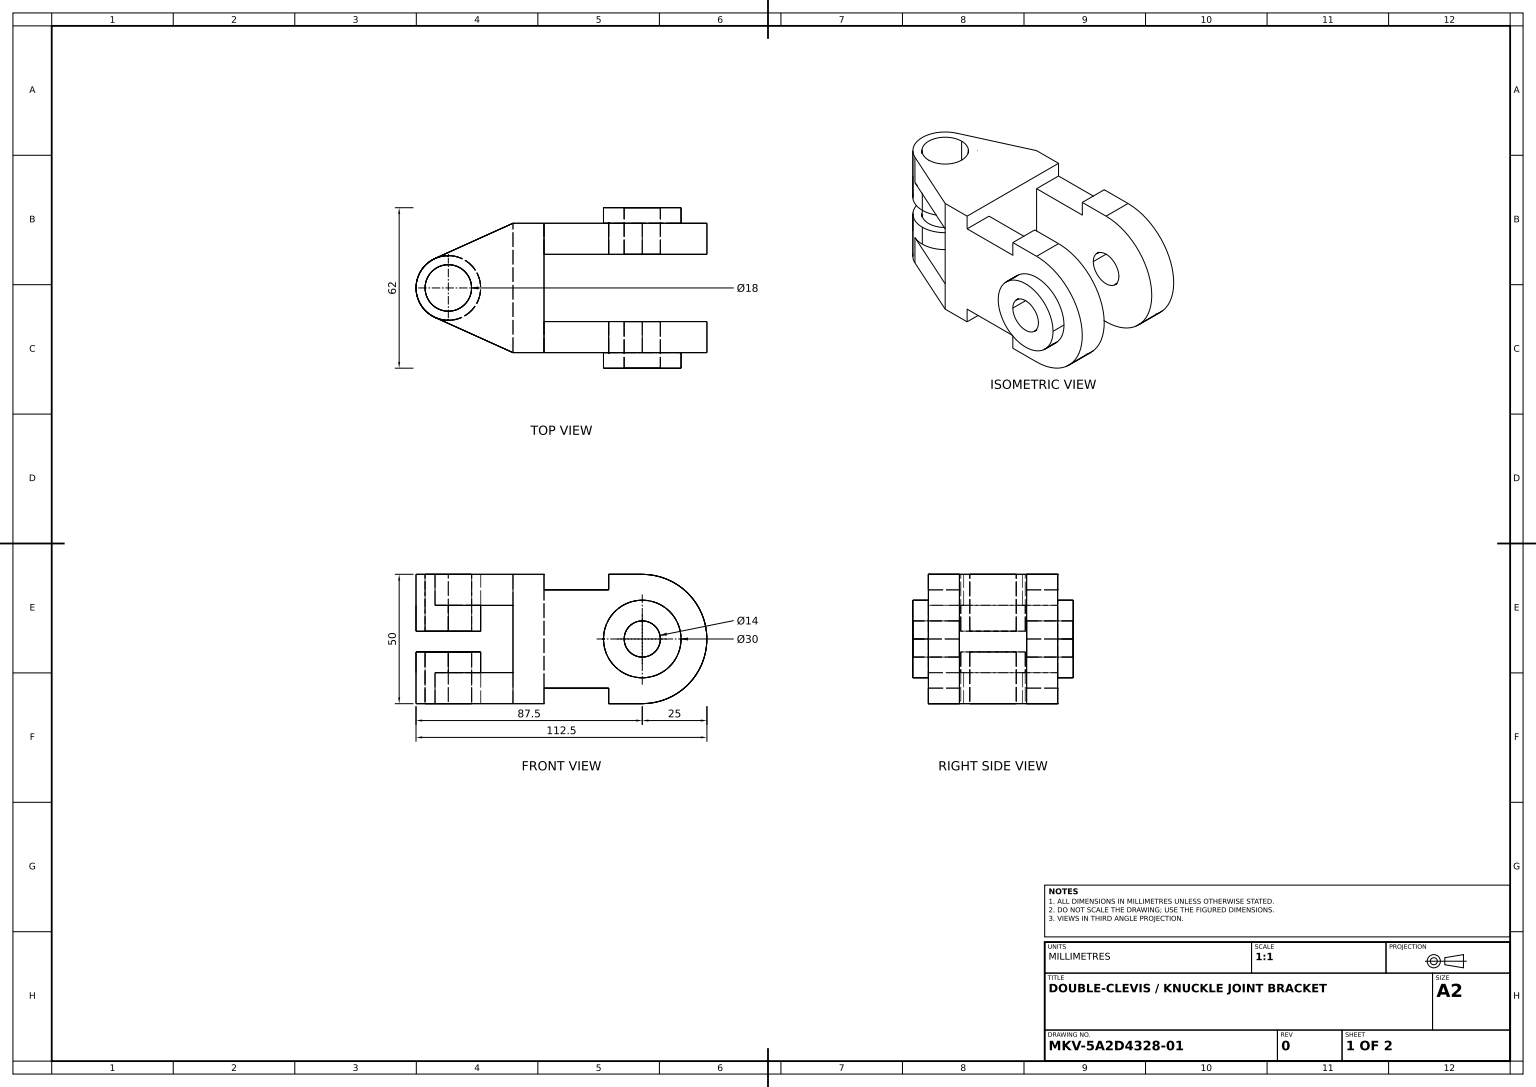
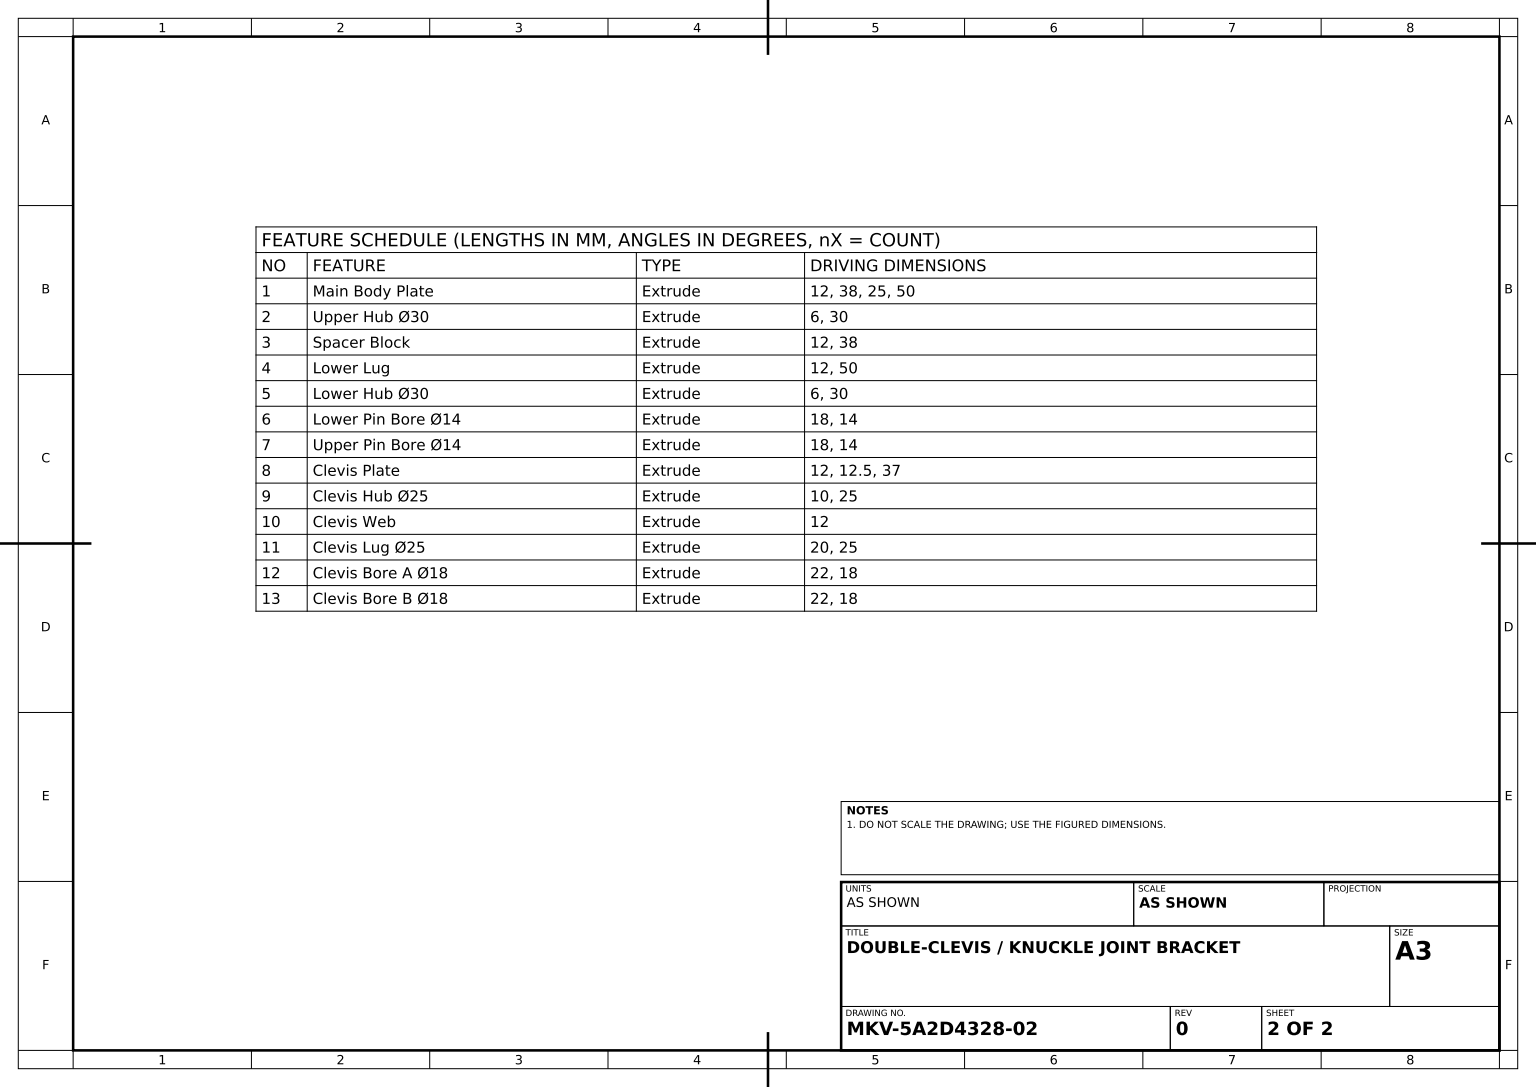
from build123d import *
from build123d.topology import SkipClean

# Parameters (mm, degrees)
MAIN_BODY_PLATE_DEPTH   = 12
UPPER_HUB_SKETCH_R      = 15
UPPER_HUB_30_DEPTH      = 6
SPACER_BLOCK_SKETCH_W   = 38
SPACER_BLOCK_SKETCH_H   = 50
SPACER_BLOCK_DEPTH      = 12
LOWER_LUG_DEPTH         = 12
LOWER_START             = 6
LOWER_HUB_SKETCH_R      = 15
LOWER_HUB_30_DEPTH      = 6
LOWER_PIN_BORE_SKETCH_R = 7
LOWER_PIN_BORE_14_DEPTH = 18
UPPER_START             = -18
UPPER_PIN_BORE_SKETCH_R = 7
UPPER_PIN_BORE_14_DEPTH = 18
CLEVIS_PLATE_DEPTH      = 12
CLEVIS_HUB_SKETCH_R     = 12.5
CLEVIS_HUB_25_DEPTH     = 10
CLEVIS_START            = -12
CLEVIS_WEB_DEPTH        = 12
CLEVIS_START_2          = -20
CLEVIS_LUG_SKETCH_R     = 12.5
CLEVIS_LUG_25_DEPTH     = 20
CLEVIS_BORE_A_SKETCH_R  = 9
CLEVIS_BORE_A_18_DEPTH  = 22
CLEVIS_START_3          = -22
CLEVIS_BORE_B_SKETCH_R  = 9
CLEVIS_BORE_B_18_DEPTH  = 22


with BuildPart() as part:
    # Main Body Profile Sketch → Main Body Plate (new body)
    with BuildSketch(Plane.XY):
        with BuildLine():
            Line((0, 0), (0, 50))
            Line((0, 50), (12, 50))
            Line((12, 50), (12, 44))
            Line((12, 44), (37, 44))
            Line((37, 44), (37, 50))
            Line((37, 50), (50, 50))
            ThreePointArc((50, 50), (75, 25), (50, 0))
            Line((50, 0), (37, 0))
            Line((37, 0), (37, 6))
            Line((37, 6), (12, 6))
            Line((12, 6), (12, 0))
            Line((12, 0), (0, 0))
        make_face()
    extrude(amount=MAIN_BODY_PLATE_DEPTH)

    # Upper Hub Sketch → Upper Hub Ø30 (add)
    with BuildSketch(Plane.XY.offset(12)):
        with Locations((50, 25)):
            Circle(UPPER_HUB_SKETCH_R)
    extrude(amount=UPPER_HUB_30_DEPTH)

    # Spacer Block Sketch → Spacer Block (add)
    with BuildSketch(Plane.ZY):
        with Locations((-19, 25)):
            Rectangle(SPACER_BLOCK_SKETCH_W, SPACER_BLOCK_SKETCH_H)
    extrude(amount=-SPACER_BLOCK_DEPTH)

    # Lower Lug Sketch → Lower Lug (add)
    with BuildSketch(Plane(origin=(0, 0, -38), x_dir=(-1, 0, 0), z_dir=(0, 0, -1))):
        with BuildLine():
            Line((-12, 44), (-37, 44))
            Line((-37, 44), (-37, 50))
            Line((-37, 50), (-50, 50))
            ThreePointArc((-50, 50), (-75, 25), (-50, 0))
            Line((-50, 0), (-37, 0))
            Line((-37, 0), (-37, 6))
            Line((-37, 6), (-12, 6))
            Line((-12, 6), (-12, 44))
        make_face()
    extrude(amount=-LOWER_LUG_DEPTH)

    # Lower Hub Sketch → Lower Hub Ø30 (add)
    with BuildSketch(Plane(origin=(0, 0, -38), x_dir=(-1, 0, 0), z_dir=(0, 0, -1)).offset(LOWER_START)):
        with Locations(Location((-50, 25, 0), (0, 0, 180))):
            Circle(LOWER_HUB_SKETCH_R)
    extrude(amount=-LOWER_HUB_30_DEPTH)

    # Lower Pin Bore Sketch → Lower Pin Bore Ø14 (cut)
    with BuildSketch(Plane(origin=(0, 0, -44), x_dir=(-1, 0, 0), z_dir=(0, 0, -1))):
        with Locations((-50, 25)):
            Circle(LOWER_PIN_BORE_SKETCH_R)
    extrude(amount=-LOWER_PIN_BORE_14_DEPTH, mode=Mode.SUBTRACT)

    # Upper Pin Bore Sketch → Upper Pin Bore Ø14 (cut)
    with BuildSketch(Plane.XY.offset(18).offset(UPPER_START)):
        with Locations(Location((50, 25, 0), (0, 0, 180))):
            Circle(UPPER_PIN_BORE_SKETCH_R)
    extrude(amount=UPPER_PIN_BORE_14_DEPTH, mode=Mode.SUBTRACT)

    # Clevis Plate Sketch → Clevis Plate (add)
    with BuildSketch(Plane(origin=(0, 50, 0), x_dir=(1, 0, 0), z_dir=(0, 1, 0))):
        with BuildLine():
            Line((0, 38), (-30.142972847, 24.392972847))
            ThreePointArc((-30.142972847, 24.392972847), (-37.5, 13), (-30.142972847, 1.607027153))
            Line((-30.142972847, 1.607027153), (0, -12))
            Line((0, -12), (0, 38))
        make_face()
    extrude(amount=-CLEVIS_PLATE_DEPTH)

    # Clevis Hub Sketch → Clevis Hub Ø25 (add)
    with SkipClean():  # the faces are left unmerged after this step: merging them gives an invalid solid
        with BuildSketch(Plane.XZ.offset(-38)):
            with Locations(Location((-25, -13, 0), (0, 0, 114.295188945))):
                Circle(CLEVIS_HUB_SKETCH_R)
        extrude(amount=CLEVIS_HUB_25_DEPTH)

    # Clevis Web Sketch → Clevis Web (add)
    with SkipClean():  # the faces are left unmerged after this step: merging them gives an invalid solid
        with BuildSketch(Plane.XZ.offset(CLEVIS_START)):
            with BuildLine():
                Line((0, -38), (0, 12))
                Line((0, 12), (-30.142972847, -1.607027153))
                ThreePointArc((-30.142972847, -1.607027153), (-18.219039913, -2.499115261), (-12.5, -13))
                ThreePointArc((-12.5, -13), (-18.219039913, -23.500884739), (-30.142972847, -24.392972847))
                Line((-30.142972847, -24.392972847), (0, -38))
            make_face()
        extrude(amount=CLEVIS_WEB_DEPTH)

    # Clevis Lug Sketch → Clevis Lug Ø25 (add)
    with SkipClean():  # the faces are left unmerged after this step: merging them gives an invalid solid
        with BuildSketch(Plane.XZ.offset(CLEVIS_START_2)):
            with Locations(Location((-25, -13, 0), (0, 0, 114.295188945))):
                Circle(CLEVIS_LUG_SKETCH_R)
        extrude(amount=CLEVIS_LUG_25_DEPTH)

    # Clevis Bore A Sketch → Clevis Bore A Ø18 (cut)
    with SkipClean():  # the faces are left unmerged after this step: merging them gives an invalid solid
        with BuildSketch(Plane(origin=(0, 50, 0), x_dir=(1, 0, 0), z_dir=(0, 1, 0))):
            with Locations(Location((-25, 13, 0), (0, 0, 270))):
                Circle(CLEVIS_BORE_A_SKETCH_R)
        extrude(amount=-CLEVIS_BORE_A_18_DEPTH, mode=Mode.SUBTRACT)

    # Clevis Bore B Sketch → Clevis Bore B Ø18 (cut)
    with SkipClean():  # the faces are left unmerged after this step: merging them gives an invalid solid
        with BuildSketch(Plane.XZ.offset(CLEVIS_START_3)):
            with Locations(Location((-25, -13, 0), (0, 0, 90))):
                Circle(CLEVIS_BORE_B_SKETCH_R)
        extrude(amount=CLEVIS_BORE_B_18_DEPTH, mode=Mode.SUBTRACT)


solid = part.part
